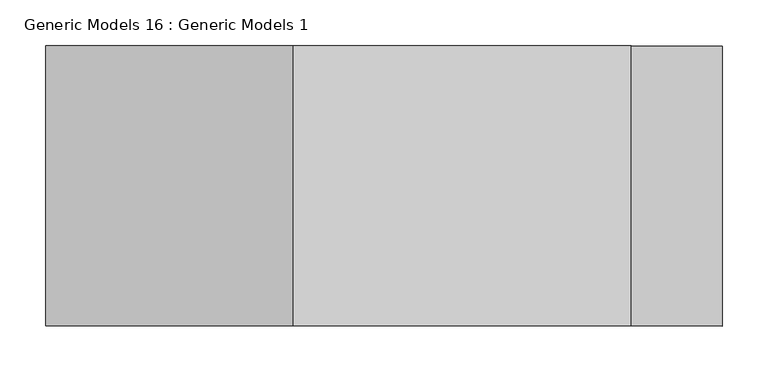
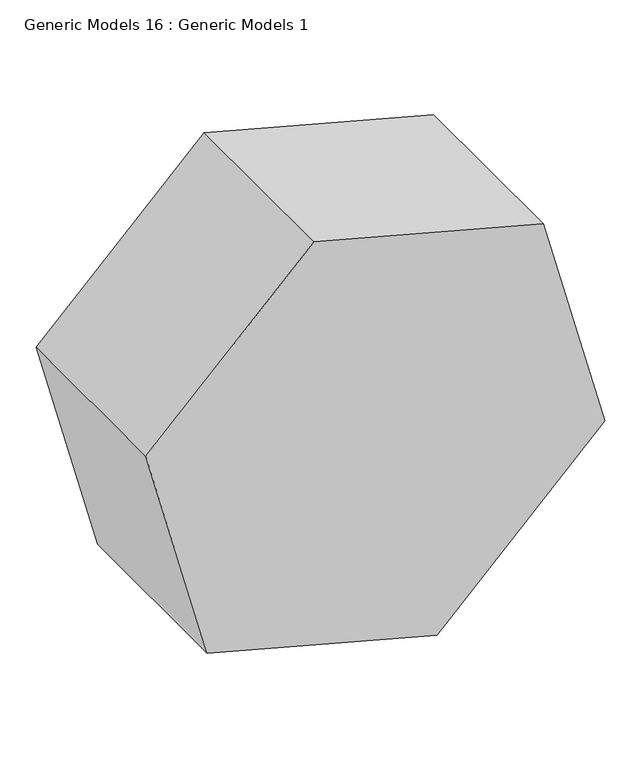
"""IFC4 building model written with IfcOpenShell, lengths in millimetres: proxy geometry, Generic Models 16 : Generic Models 1."""

from ifc_helpers import new_model, si_unit, frame, origin, place, context, project, spatial, polyline, outline, extrude, source, transform, mapped, element, save


def generic_models_16_generic_models_1_a0735545(model_context):
    return source(origin(), model_context, "Body", "SweptSolid", [
        extrude(outline(polyline([(904.7566299, 6993.0198357), (1003.366686, 6625.0020959), (733.9590024, 6355.5944123), (365.9412626, 6454.2044685), (267.3312064, 6822.2222083), (536.73889, 7091.6298919), (904.7566299, 6993.0198357)])), frame((0.0, -9086.6225464, 0.0), z_axis=(0.0, 1.0, 0.0), x_axis=(0.0, 0.0, 1.0)), (0.0, 0.0, 1.0), 304.8),
    ])


if __name__ == "__main__":
    model = new_model("IFC4")
    model_context = context("Model", 3, world=origin())
    ifc_project = project(units=[si_unit("LENGTHUNIT", "METRE", prefix="MILLI")], contexts=[model_context])
    site = spatial("IfcSite", under=ifc_project)
    building = spatial("IfcBuilding", under=site)
    placement = place(None, origin())
    generic_models_16_generic_models_1_shape = generic_models_16_generic_models_1_a0735545(model_context)
    element("IfcBuildingElementProxy", 1, Name="Generic Models 16 : Generic Models 1", ObjectType="Generic Models 16 : Generic Models 1", at=placement, inside=building, context=model_context, shape_type="MappedRepresentation", body=[
        mapped(generic_models_16_generic_models_1_shape, transform((0.0, 0.0, 0.0), x_axis=(1.0, 0.0, 0.0), y_axis=(0.0, 1.0, 0.0), z_axis=(0.0, 0.0, 1.0))),
    ])
    save(model, "model.ifc")

# Revit data of these elements
# Element 1 (IfcBuildingElementProxy, "Generic Models 16 : Generic Models 1")
#   Materials on its faces: "Brick, Common"
# Materials
#   "Brick, Common": class "Masonry", colour RGB 170 98 104, transparency 0, Description = "Common brick", Cost = 0
